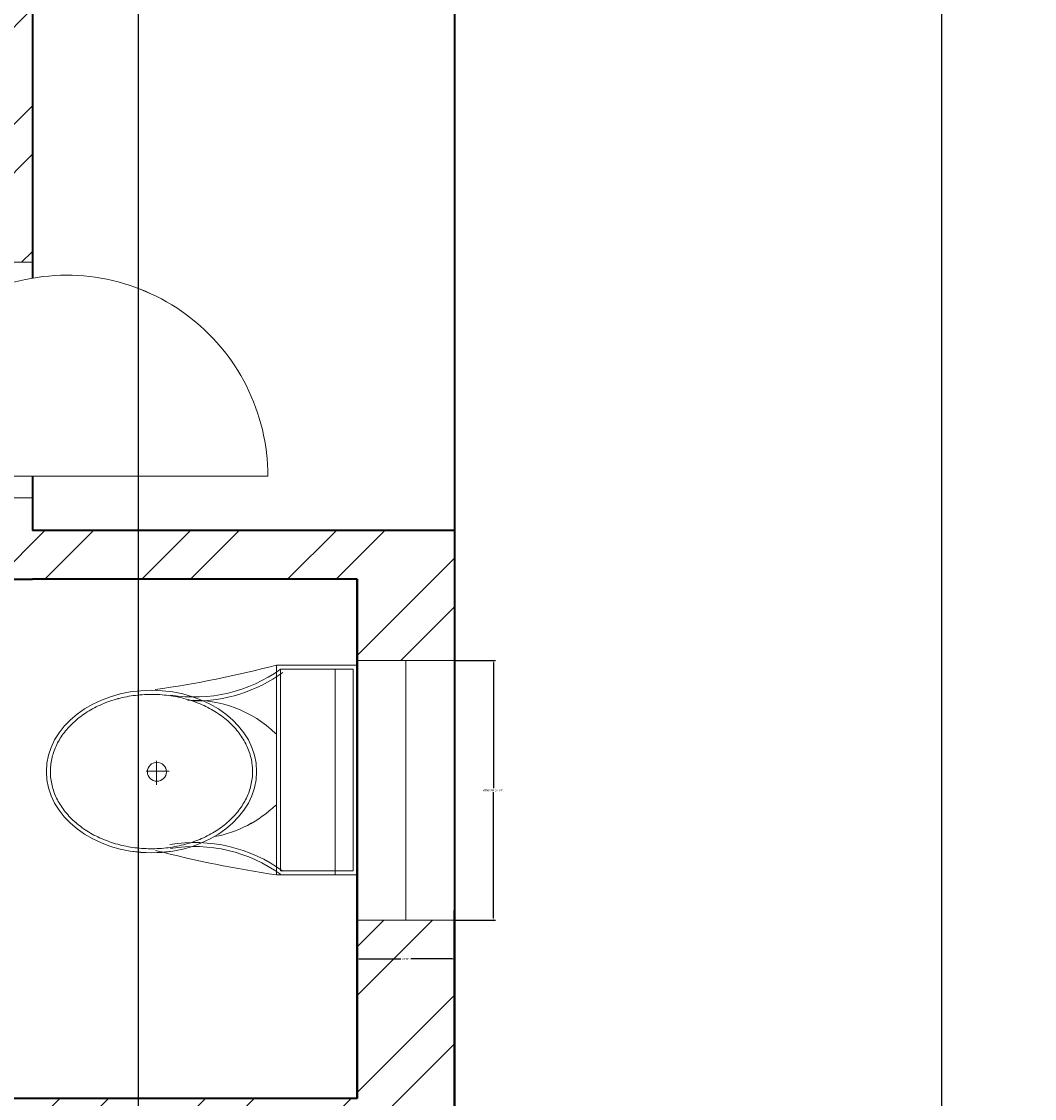
# Model space of a CAD drawing. Units: inches. Extents: x 2120 to 4013, y 1390 to 3019.
# Tile 45 of 59: x 2970 to 3063, y 2165 to 2265. Entities that reach past the tile are written whole.
import ezdxf

# ---------------------------------------------------------------- set-up
doc = ezdxf.new("R2010")
doc.units = ezdxf.units.IN
for name, color, linetype, lineweight in [('A-ANNO-DIMS', 2, 'Continuous', 18), ('A-DOOR', 3, 'Continuous', 18), ('A-FLOR-FIXT', 9, 'Continuous', 18), ('A-GLAZ', 4, 'Continuous', 18), ('A-WALL', 7, 'Continuous', 35), ('A-WALL-PATT', 252, 'Continuous', 13)]:
    doc.layers.add(name, color=color, linetype=linetype, lineweight=lineweight)
doc.styles.get("Standard").update_dxf_attribs({"font": 'arial.ttf'})
doc.dimstyles.get("Standard").update_dxf_attribs({"dimtxt": 0.18, "dimasz": 0.18, "dimexe": 0.18, "dimexo": 0.0625, "dimgap": 0.09, "dimtad": 0, "dimtih": 1, "dimtoh": 1, "dimdec": 4, "dimzin": 0, "dimdsep": 46, "dimtxsty": 'Standard', "dimcen": 0.09, "dimadec": 0, "dimazin": 0, "dimtfac": 1, "dimtdec": 4, "dimtofl": 0, "dimtmove": 0, "dimatfit": 3, "dimfxl": 1, "dimtolj": 1, "dimtzin": 0, "dimarcsym": 0})

# ---------------------------------------------------------------- blocks, each defined once
blk = doc.blocks.new('A$C31115884')
for p, q in [((257.5, 466.4), (257.5, 523.2)), ((283.1, 497.7), (223.4, 497.7)), ((0, 200), (0, 0)), ((520, 200), (0, 200)), ((10, 190), (10, 10)), ((510, 190), (10, 190)), ((510, 10), (510, 190)), ((520, 0), (520, 200)), ((510, 54.5), (0, 54.5)), ((10, 10), (510, 10)), ((0, 0), (520, 0))]:
    blk.add_line(p, q)
blk.add_circle((255.6, 496.4), 23.6)
for centre, radius, start, end in [((2777.7, -204.6), 2807, 165.4549, 171.7133), ((3237, 905), 2807, 188.2867, 194.5451), ((-294.5, 403.3), 364.7, 324.2091, 9.3499), ((-294.5, 403.3), 374.7, 324.2091, 9.3499), ((805.8, 403.3), 364.7, 170.6501, 215.7909), ((139.5, 406.2), 293.5, 315.8436, 2.6563), ((805.8, 403.3), 374.7, 179.2036, 215.7909), ((383.6, 406.2), 293.5, 190.2774, 224.1564)]:
    blk.add_arc(centre, radius, start, end)
blk.add_ellipse((256.2, 509.9), major_axis=(0, -260.7), ratio=0.772727)
blk.add_open_spline([(256.2, 259.2), (263.1, 259.2), (270, 259.7), (287.8, 262.3), (298.7, 265.1), (319.9, 273.1), (330.2, 278.4), (350.1, 291.1), (359.7, 298.7), (377.7, 315.9), (386.2, 325.5), (401.7, 346.6), (408.8, 358.1), (421.3, 382.5), (426.8, 395.5), (435.9, 422.4), (439.5, 436.4), (444.8, 465.1), (446.5, 479.7), (447.9, 509.2), (447.6, 524), (445, 553.3), (442.7, 567.8), (436.3, 596), (432.1, 609.7), (421.9, 636), (416, 648.6), (402.5, 672.1), (395, 683), (378.6, 703), (369.8, 712.1), (351.1, 728), (341.3, 734.8), (320.9, 746.2), (310.4, 750.7), (288.9, 757.3), (278, 759.4), (256, 761), (245, 760.6), (223.1, 757.2), (212.3, 754.3), (191.1, 746.1), (180.8, 740.7), (160.9, 727.8), (151.4, 720.1), (133.5, 702.7), (125.1, 693), (109.6, 671.7), (102.6, 660.2), (90.2, 635.7), (84.9, 622.7), (76, 595.6), (72.4, 581.6), (67.2, 552.9), (65.6, 538.2), (64.4, 508.8), (64.8, 494), (67.5, 464.7), (69.9, 450.2), (76.6, 422), (80.8, 408.3), (91.1, 382.2), (97.2, 369.7), (110.8, 346.3), (118.4, 335.4), (134.8, 315.6), (143.7, 306.7), (162.4, 290.9), (172.3, 284.2), (192.8, 273), (203.3, 268.6), (224.8, 262.2), (235.8, 260.2), (249.9, 259.3), (253, 259.2), (256.2, 259.2)], degree=3, knots=[0, 0, 0, 0, 0.110105, 0.110105, 0.285049, 0.285049, 0.459994, 0.459994, 0.634938, 0.634938, 0.809882, 0.809882, 0.984827, 0.984827, 1.159771, 1.159771, 1.334715, 1.334715, 1.50966, 1.50966, 1.684604, 1.684604, 1.859549, 1.859549, 2.034493, 2.034493, 2.209437, 2.209437, 2.384382, 2.384382, 2.559326, 2.559326, 2.73427, 2.73427, 2.909215, 2.909215, 3.084159, 3.084159, 3.259103, 3.259103, 3.434048, 3.434048, 3.608992, 3.608992, 3.783936, 3.783936, 3.958881, 3.958881, 4.133825, 4.133825, 4.30877, 4.30877, 4.483714, 4.483714, 4.658658, 4.658658, 4.833603, 4.833603, 5.008547, 5.008547, 5.183491, 5.183491, 5.358436, 5.358436, 5.53338, 5.53338, 5.708324, 5.708324, 5.883269, 5.883269, 6.058213, 6.058213, 6.233158, 6.233158, 6.283185, 6.283185, 6.283185, 6.283185])
blk = doc.blocks.new('DOOR-SWING-24IN-106p92DEG')
for p, q in [((4.5, 21.786), (0, 21.786)), ((0, 21.786), (2.25, 21.786)), ((2.25, 21.786), (2.25, 19.786)), ((2.25, 0), (2.25, 2)), ((2.25, 2), (26.25, 2)), ((0, 0), (4.5, 0)), ((4.5, 0), (2.25, 0))]:
    blk.add_line(p, q)
blk.add_arc((7.66, 2), 18.59, 0, 106.91809)
blk = doc.blocks.new('WIN-PLAN-24IN-04')
for p, q in [((0, 24), (9, 24)), ((9, 24), (4.5, 24)), ((4.5, 24), (4.5, 0)), ((9, 24), (9, 24)), ((4.5, 0), (0, 0)), ((0, 0), (9, 0))]:
    blk.add_line(p, q)
blk = doc.blocks.new('*D183')
at = {"layer": 'A-ANNO-DIMS', "color": 0, "lineweight": -2, "transparency": 16777216}
for p, q in [((3009.796, 2205.523), (3013.513, 2205.523)), ((3013.333, 2205.343), (3013.333, 2193.706)), ((3013.333, 2181.703), (3013.333, 2193.34)), ((3009.796, 2181.523), (3013.513, 2181.523))]:
    blk.add_line(p, q, dxfattribs=at)
at = {"layer": 'A-ANNO-DIMS', "color": 0, "transparency": 16777216}
for points in [[(3013.303, 2205.343), (3013.363, 2205.343), (3013.333, 2205.523)], [(3013.303, 2181.703), (3013.363, 2181.703), (3013.333, 2181.523)]]:
    blk.add_solid(points, dxfattribs=at)
at = {"layer": 'Defpoints', "color": 0, "transparency": 16777216}
for p in [(3009.733, 2205.523), (3013.333, 2205.523), (3009.733, 2181.523)]:
    blk.add_point(p, dxfattribs=at)
at = {"layer": 'A-ANNO-DIMS', "color": 0, "transparency": 16777216, "insert": (3013.333, 2193.523), "char_height": 0.18, "attachment_point": 5}
blk.add_mtext('\\A1;WINDOW 24 TYP.', dxfattribs=at)
blk = doc.blocks.new('*D184')
at = {"layer": 'A-ANNO-DIMS', "color": 0, "lineweight": -2, "transparency": 16777216}
for p, q in [((3000.733, 2181.46), (3000.733, 2177.743)), ((3009.733, 2181.46), (3009.733, 2177.743)), ((3000.913, 2177.923), (3004.775, 2177.923)), ((3009.553, 2177.923), (3005.691, 2177.923))]:
    blk.add_line(p, q, dxfattribs=at)
at = {"layer": 'A-ANNO-DIMS', "color": 0, "transparency": 16777216}
for points in [[(3000.913, 2177.953), (3000.913, 2177.893), (3000.733, 2177.923)], [(3009.553, 2177.953), (3009.553, 2177.893), (3009.733, 2177.923)]]:
    blk.add_solid(points, dxfattribs=at)
at = {"layer": 'Defpoints', "color": 0, "transparency": 16777216}
for p in [(3000.733, 2181.523), (3009.733, 2181.523), (3009.733, 2177.923)]:
    blk.add_point(p, dxfattribs=at)
at = {"layer": 'A-ANNO-DIMS', "color": 0, "transparency": 16777216, "insert": (3005.233, 2177.923), "char_height": 0.18, "attachment_point": 5}
blk.add_mtext('\\A1;9 TYP.', dxfattribs=at)
blk = doc.blocks.new('*D212')
at = {"layer": 'A-ANNO-DIMS', "color": 0, "lineweight": -2, "transparency": 16777216}
for p, q in [((3009.796, 2352.531), (3054.913, 2352.531)), ((3054.733, 2352.351), (3054.733, 1947.713)), ((3054.733, 1542.711), (3054.733, 1947.349)), ((3009.796, 1542.531), (3054.913, 1542.531))]:
    blk.add_line(p, q, dxfattribs=at)
at = {"layer": 'A-ANNO-DIMS', "color": 0, "transparency": 16777216}
for points in [[(3054.703, 2352.351), (3054.763, 2352.351), (3054.733, 2352.531)], [(3054.703, 1542.711), (3054.763, 1542.711), (3054.733, 1542.531)]]:
    blk.add_solid(points, dxfattribs=at)
at = {"layer": 'Defpoints', "color": 0, "transparency": 16777216}
for p in [(3009.733, 2352.531), (3009.733, 1542.531), (3054.733, 1542.531)]:
    blk.add_point(p, dxfattribs=at)
at = {"layer": 'A-ANNO-DIMS', "color": 0, "transparency": 16777216, "insert": (3054.733, 1947.531), "char_height": 0.18, "attachment_point": 5}
blk.add_mtext('\\A1;810', dxfattribs=at)
blk = doc.blocks.new('*D217')
at = {"layer": 'A-ANNO-DIMS', "color": 0, "lineweight": -2, "transparency": 16777216}
for p, q in [((3071.672, 2352.531), (2980.308, 2352.531)), ((2980.488, 2352.351), (2980.488, 1947.713)), ((2980.488, 1542.711), (2980.488, 1947.349)), ((3305.672, 1542.531), (2980.308, 1542.531))]:
    blk.add_line(p, q, dxfattribs=at)
at = {"layer": 'A-ANNO-DIMS', "color": 0, "transparency": 16777216}
for points in [[(2980.458, 2352.351), (2980.518, 2352.351), (2980.488, 2352.531)], [(2980.458, 1542.711), (2980.518, 1542.711), (2980.488, 1542.531)]]:
    blk.add_solid(points, dxfattribs=at)
at = {"layer": 'Defpoints', "color": 0, "transparency": 16777216}
for p in [(2980.488, 2352.531), (3071.735, 2352.531), (3305.735, 1542.531)]:
    blk.add_point(p, dxfattribs=at)
at = {"layer": 'A-ANNO-DIMS', "color": 0, "transparency": 16777216, "insert": (2980.488, 1947.531), "char_height": 0.18, "attachment_point": 5}
blk.add_mtext('\\A1;810', dxfattribs=at)

msp = doc.modelspace()

# ---------------------------------------------------------------- hatches: boundary and pattern name
at = {"layer": 'A-WALL-PATT'}
h = msp.add_hatch(dxfattribs=at)
h.set_pattern_fill('ANSI32', color=256)
h.paths.add_polyline_path([(2271.7331, 2122.6377), (2262.7331, 2122.6377), (2262.7331, 2040.3893), (2267.2331, 2040.3893), (2271.7331, 2040.3893), (2271.7331, 2044.8856), (2271.7331, 2070.531), (2391.7331, 2070.531), (2391.7331, 1926.5306), (2388.3993, 1926.5306), (2388.3993, 1922.531), (2395.7331, 1922.531), (2395.7331, 1992.531), (2400.4511, 1992.531), (2400.4511, 1997.0306), (2395.7331, 1997.0306), (2395.7331, 2070.531), (2443.7331, 2070.531), (2443.7331, 2046.1368), (2448.2331, 2046.1368), (2448.2331, 2070.531), (2580.2331, 2070.531), (2580.2331, 1997.0306), (2492.9076, 1997.0306), (2492.9076, 1992.531), (2580.2331, 1992.531), (2580.2331, 1983.9368), (2589.2331, 1983.9368), (2589.2331, 2070.531), (2589.2331, 2075.0306), (2396.2331, 2075.0306), (2396.2331, 2184.3565), (2393.9831, 2184.3565), (2391.7331, 2184.3565), (2391.7331, 2075.0306), (2271.7331, 2075.0306)])
h.paths.add_polyline_path([(2724.7331, 2138.0306), (2628.7331, 2138.0306), (2628.7331, 2070.5306), (2628.7331, 2067.0987), (2633.2331, 2067.0987), (2637.7331, 2067.0987), (2637.7331, 2070.531), (2657.3413, 2070.531), (2657.3413, 2079.5306), (2637.7331, 2079.5306), (2637.7331, 2129.031), (2715.7331, 2129.031), (2715.7331, 2079.5306), (2698.0378, 2079.5306), (2698.0378, 2070.531), (2715.7331, 2070.531), (2715.7331, 2012.1531), (2720.2331, 2012.1531), (2724.7331, 2012.1531)])
h.paths.add_polyline_path([(2724.7331, 2213.031), (2831.3209, 2213.031), (2831.3209, 2215.281), (2831.3209, 2217.5306), (2724.7331, 2217.5306), (2724.7331, 2343.531), (2751.8755, 2343.531), (2751.8755, 2352.5306), (2715.7331, 2352.5306), (2715.7331, 2138.031), (2724.7331, 2138.031)])
h.paths.add_polyline_path([(2902.53, 2352.5306), (2811.8755, 2352.5306), (2811.8755, 2343.531), (2867.2331, 2343.531), (2867.2331, 2217.5306), (2863.6364, 2217.5306), (2863.6364, 2213.031), (2871.7331, 2213.031), (2871.7331, 2217.531), (2871.7331, 2343.531), (2902.53, 2343.531)])
h.paths.add_polyline_path([(3009.7331, 2352.5306), (2938.53, 2352.5306), (2938.53, 2343.531), (2966.2331, 2343.531), (2966.2331, 2242.3281), (2968.4831, 2242.3281), (2970.7331, 2242.3281), (2970.7331, 2343.531), (3009.7331, 2343.531)])
h.paths.add_polyline_path([(3009.7331, 2217.5306), (2970.7331, 2217.5306), (2970.7331, 2220.5422), (2968.4831, 2220.5422), (2966.2331, 2220.5422), (2966.2331, 2217.5306), (2911.7752, 2217.5306), (2907.7331, 2217.5306), (2907.7331, 2213.0306), (2907.7331, 2194.9663), (2912.2331, 2194.9663), (2912.2331, 2213.031), (2970.7331, 2213.031), (3000.7331, 2213.031), (3000.7331, 2205.523), (3009.7331, 2205.523)])
h.paths.add_polyline_path([(3009.7331, 2181.5227), (3000.7331, 2181.5227), (3000.7331, 2165.0306), (2912.2331, 2165.0306), (2912.2331, 2170.8202), (2907.7331, 2170.8202), (2907.7331, 2165.0306), (2899.5169, 2165.0306), (2899.5169, 2162.7806), (2899.5169, 2160.531), (2907.7331, 2160.531), (2907.7331, 2137.3432), (2912.2331, 2137.3432), (2912.2331, 2160.531), (3000.7331, 2160.531), (3000.7331, 2150.4993), (3009.7331, 2150.4993)])
h.paths.add_polyline_path([(3009.7331, 2126.499), (3005.2331, 2126.499), (3000.7331, 2126.499), (3000.7331, 2112.5306), (2912.2331, 2112.5306), (2912.2331, 2115.6036), (2907.7331, 2115.6036), (2907.7331, 2108.031), (3000.7331, 2108.031), (3000.7331, 2084.7256), (3009.7331, 2084.7256)], flags=17)
h.paths.add_polyline_path([(3009.7331, 1971.531), (3009.7331, 2024.7253), (3000.7331, 2024.7253), (3000.7331, 2006.4153), (3000.7331, 1971.5306), (2864.2331, 1971.5306), (2864.2331, 2160.531), (2868.0522, 2160.531), (2868.0522, 2165.0306), (2859.7331, 2165.0306), (2859.7331, 1971.5306), (2724.7331, 1971.5306), (2724.7331, 1977.7012), (2715.7331, 1977.7012), (2715.7331, 1962.5306), (2715.7331, 1950.9035), (2720.2331, 1950.9035), (2724.7331, 1950.9035), (2724.7331, 1962.531), (2855.2331, 1962.531), (2859.7331, 1962.531), (2859.7331, 1835.031), (2864.2331, 1834.8158), (2864.2331, 1962.531), (2958.7331, 1962.531), (2958.7331, 1937.0925), (2963.2331, 1937.0925), (2963.2331, 1962.531), (3000.7331, 1962.531), (3009.7331, 1962.531)])
h.paths.add_polyline_path([(2724.7331, 1728.531), (2822.7164, 1728.531), (2822.7164, 1733.0306), (2724.7331, 1733.0306), (2724.7331, 1779.3416), (2715.7331, 1779.3416), (2715.7331, 1581.531), (2753.02, 1581.531), (2753.02, 1586.031), (2753.02, 1590.5306), (2724.7331, 1590.5306)])
h.paths.add_polyline_path([(2864.2331, 1590.531), (2864.2331, 1787.031), (2868.4075, 1787.031), (2868.4075, 1791.5306), (2859.7331, 1791.5306), (2859.7331, 1739.0306), (2859.7331, 1733.0306), (2854.3125, 1733.0306), (2854.3125, 1728.531), (2859.7331, 1728.531), (2859.7331, 1590.5306), (2813.02, 1590.5306), (2813.02, 1581.531), (2868.4123, 1581.531), (2868.4123, 1583.781), (2868.4123, 1586.0306), (2864.2331, 1586.0306)])
h.paths.add_polyline_path([(3009.7331, 1754.6619), (3000.7331, 1754.6619), (3000.7331, 1739.0306), (2912.2331, 1739.0306), (2912.2331, 1742.2257), (2907.7331, 1742.2257), (2907.7331, 1739.0306), (2907.7331, 1734.531), (3000.7331, 1734.531), (3000.7331, 1590.5306), (3000.7331, 1586.0306), (2971.3921, 1586.0306), (2971.3921, 1581.531), (3009.7331, 1581.531)])
h.paths.add_polyline_path([(2911.3921, 1583.781), (2911.3921, 1586.0306), (2891.2138, 1586.0306), (2891.2138, 1581.531), (2911.3921, 1581.531)])
h.paths.add_polyline_path([(3009.7331, 1799.8422), (3000.7331, 1799.8422), (3000.7331, 1791.5306), (2912.2331, 1791.5306), (2912.2331, 1796.3264), (2909.9831, 1796.3264), (2907.7331, 1796.3264), (2907.7331, 1791.5306), (2902.7033, 1791.5306), (2902.7033, 1787.031), (2907.7331, 1787.031), (2907.7331, 1761.1622), (2912.2331, 1761.1622), (2912.2331, 1787.031), (3000.7331, 1787.031), (3000.7331, 1778.6622), (3009.7331, 1778.6622)])
h.paths.add_polyline_path([(3009.7331, 1839.5306), (2963.2331, 1839.5306), (2963.2331, 1842.8629), (2960.9831, 1842.8629), (2958.7331, 1842.8629), (2958.7331, 1839.5306), (2907.7331, 1839.5306), (2907.7331, 1814.4599), (2912.2331, 1814.4599), (2912.2331, 1835.031), (3000.7331, 1835.031), (3000.7331, 1823.8425), (3009.7331, 1823.8425), (3009.7331, 1835.031)])
h.paths.add_polyline_path([(2963.2331, 1901.0922), (2960.9831, 1901.0922), (2958.7331, 1901.0922), (2958.7331, 1862.8843), (2963.2331, 1862.8843)], flags=17)
h.paths.add_polyline_path([(2724.7331, 1891.9826), (2724.7331, 1914.3416), (2715.7331, 1914.3416), (2715.7331, 1783.8416), (2637.7331, 1783.8416), (2637.7331, 1914.3416), (2628.7331, 1914.3416), (2624.7701, 1914.3416), (2624.7701, 1909.8416), (2624.7701, 1905.3419), (2628.7331, 1905.3419), (2628.7331, 1876.9915), (2628.7331, 1779.3419), (2637.7331, 1779.3419), (2715.7331, 1779.3419), (2724.7331, 1779.3419), (2724.7331, 1835.031)])
h.paths.add_polyline_path([(2637.7331, 1731.531), (2637.7331, 1779.3416), (2628.7331, 1779.3416), (2628.7331, 1731.5306), (2589.2331, 1731.5306), (2535.9814, 1731.5306), (2496.7331, 1731.5306), (2496.7331, 1725.6876), (2498.9831, 1725.6876), (2501.2331, 1725.6876), (2501.2331, 1727.031), (2628.7331, 1727.031), (2628.7331, 1680.4203), (2628.7331, 1590.5306), (2628.7331, 1586.0306), (2604.1361, 1586.0306), (2604.1361, 1581.531), (2637.7331, 1581.531), (2637.7331, 1590.531)])

# ---------------------------------------------------------------- linework, layer by layer
at = {"layer": 'A-WALL'}
for p, q in [((3009.7331, 2352.531), (3009.7331, 2075.031)), ((3009.7331, 2352.5306), (3009.7331, 2075.0306)), ((2970.7331, 2343.531), (2970.7331, 2240.8622)), ((2970.7331, 2343.5306), (2970.7331, 2240.8619)), ((2970.7331, 2222.5425), (2970.7331, 2217.531)), ((2970.7331, 2222.5422), (2970.7331, 2217.5306)), ((3009.7331, 2217.531), (2970.7331, 2217.531)), ((3009.7331, 2217.5306), (2970.7331, 2217.5306)), ((2912.2331, 2213.031), (2970.7331, 2213.031)), ((2912.2331, 2213.0306), (2970.7331, 2213.0306)), ((3000.7331, 2213.031), (2970.7331, 2213.031)), ((3000.7331, 2213.0306), (2970.7331, 2213.0306)), ((3000.7331, 2182.408), (3000.7331, 2213.031)), ((3000.7331, 2213.031), (3000.7331, 2165.031)), ((3000.7331, 2182.4077), (3000.7331, 2213.0306)), ((3000.7331, 2213.0306), (3000.7331, 2165.0306)), ((3000.7331, 2165.031), (3000.7331, 2182.408)), ((3000.7331, 2165.0306), (3000.7331, 2182.4077)), ((3009.7331, 1971.531), (3009.7331, 2182.408)), ((3009.7331, 1971.5306), (3009.7331, 2182.4077)), ((3000.7331, 2165.031), (2912.2331, 2165.031)), ((3000.7331, 2165.0306), (2912.2331, 2165.0306))]:
    msp.add_line(p, q, dxfattribs=at)

# ---------------------------------------------------------------- block references
at = {"layer": 'A-DOOR'}
for p in [(2966.2331, 2220.5425), (2966.2331, 2220.5422)]:
    msp.add_blockref('DOOR-SWING-24IN-106p92DEG', p, dxfattribs=at)
at = {"layer": 'A-FLOR-FIXT', "xscale": 0.0372717239612423, "yscale": 0.0372717239612423, "zscale": 0.0372717239612423, "rotation": 89.99999999999999}
for p in [(3000.7331, 2185.7042), (3000.7331, 2185.7039)]:
    msp.add_blockref('A$C31115884', p, dxfattribs=at)
at = {"layer": 'A-GLAZ'}
for p in [(3000.7331, 2181.523), (3000.7331, 2181.5227)]:
    msp.add_blockref('WIN-PLAN-24IN-04', p, dxfattribs=at)

# ---------------------------------------------------------------- dimensions: what is measured, and where the dimension line sits
at = {"layer": 'A-ANNO-DIMS'}
for base, p1, p2, picture, middle in [((2980.4877, 2352.531), (3305.7347, 1542.531), (3071.7347, 2352.531), '*D217', (2980.4877, 1947.531)), ((3054.7331, 1542.531), (3009.7331, 2352.531), (3009.7331, 1542.531), '*D212', (3054.7331, 1947.531))]:
    dim = msp.add_linear_dim(base=base, p1=p1, p2=p2, angle=90, dimstyle='Standard', override={"dimdec": 0, "dimlfac": 1, "dimrnd": 0, "dimzin": 0, "dimdsep": 46, "dimlunit": 2}, dxfattribs=at)
    dim.commit()
    dim.dimension.update_dxf_attribs({"geometry": picture, "text_midpoint": middle})
dim = msp.add_linear_dim(base=(3013.3331, 2205.523), p1=(3009.7331, 2181.523), p2=(3009.7331, 2205.523), angle=90, text='WINDOW <> TYP.', dimstyle='Standard', override={"dimdec": 0, "dimlfac": 1, "dimrnd": 0, "dimzin": 0, "dimdsep": 46, "dimlunit": 2}, dxfattribs=at)
dim.commit()
dim.dimension.update_dxf_attribs({"geometry": '*D183', "text_midpoint": (3013.3331, 2193.523)})
dim = msp.add_linear_dim(base=(3009.7331, 2177.923), p1=(3000.7331, 2181.523), p2=(3009.7331, 2181.523), text='<> TYP.', dimstyle='Standard', override={"dimdec": 0, "dimlfac": 1, "dimrnd": 0, "dimzin": 0, "dimdsep": 46, "dimlunit": 2}, dxfattribs=at)
dim.commit()
dim.dimension.update_dxf_attribs({"geometry": '*D184', "text_midpoint": (3005.2331, 2177.923)})

doc.saveas('drawing.dxf')
